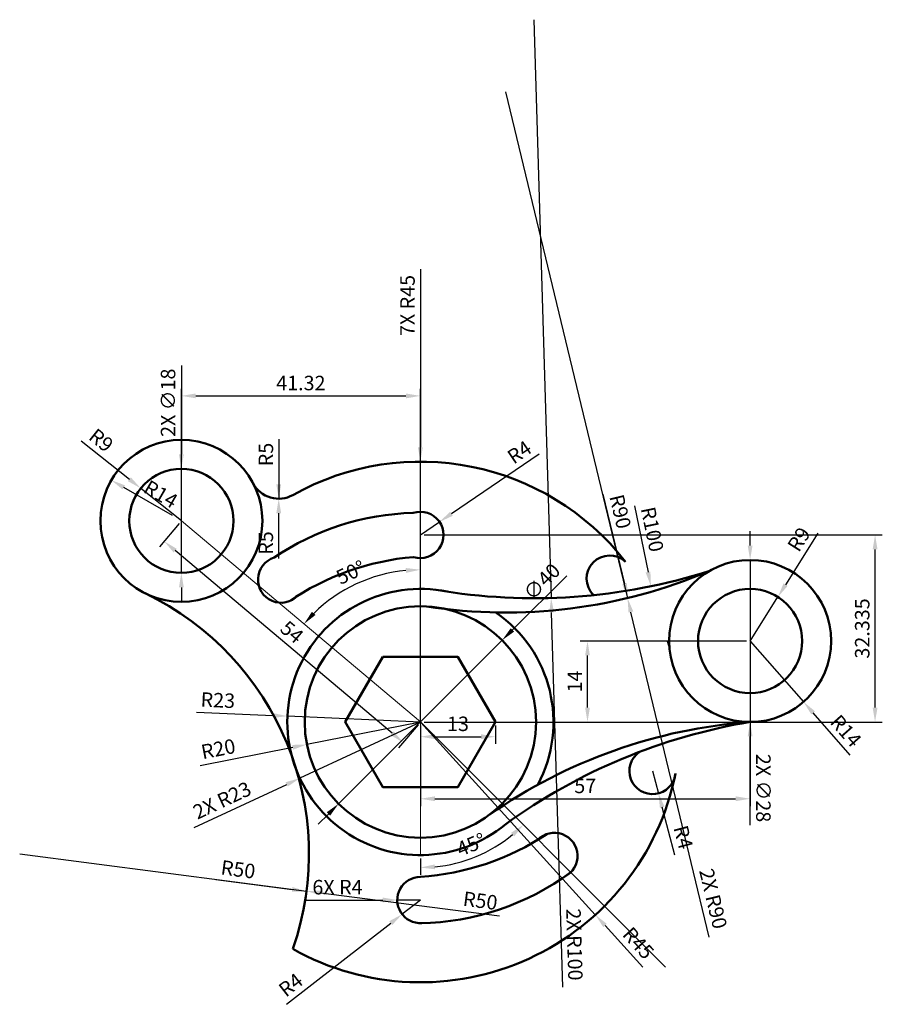
# Model space of a CAD drawing. Units: millimetres. Extents: x 2630 to 2779, y 1501 to 1671.
import ezdxf

# ---------------------------------------------------------------- set-up
doc = ezdxf.new("R2010")
doc.units = ezdxf.units.MM
for name, color, linetype, lineweight in [('M-CONS', 8, 'Continuous', 18), ('M-DIMS', 2, 'Continuous', 25), ('M-OUTL', 7, 'Continuous', 50)]:
    doc.layers.add(name, color=color, linetype=linetype, lineweight=lineweight)
doc.styles.get("Standard").update_dxf_attribs({"font": 'arial.ttf'})
doc.dimstyles.new('ISO-25', dxfattribs={"dimtxt": 2.5, "dimasz": 2.5, "dimexe": 1.25, "dimexo": 0.625, "dimtad": 1, "dimtxsty": 'Standard', "dimcen": 2.5, "dimadec": 0, "dimazin": 0, "dimtfac": 1, "dimtmove": 0, "dimatfit": 3, "dimfxl": 1, "dimarcsym": 0})

# ---------------------------------------------------------------- blocks, each defined once
blk = doc.blocks.new('*D1')
at = {"layer": 'Defpoints', "color": 0, "transparency": 16777216}
for p in [(2658.07, 1584.79), (2655.1, 1581.25), (2699.39, 1550.02)]:
    blk.add_point(p, dxfattribs=at)
at = {"layer": 'M-DIMS', "color": 0, "lineweight": -2, "transparency": 16777216}
for p, q in [((2657.67, 1584.31), (2654.29, 1580.3)), ((2694.5, 1548.09), (2657.01, 1579.64)), ((2698.99, 1549.54), (2695.61, 1545.53))]:
    blk.add_line(p, q, dxfattribs=at)
at = {"layer": 'M-DIMS', "color": 0, "transparency": 16777216}
for points in [[(2657.28, 1579.96), (2656.74, 1579.32), (2655.1, 1581.25)], [(2694.77, 1548.41), (2694.23, 1547.77), (2696.41, 1546.48)]]:
    blk.add_solid(points, dxfattribs=at)
at = {"layer": 'M-DIMS', "color": 0, "transparency": 16777216, "insert": (2676.98, 1565.32), "char_height": 2.5, "attachment_point": 5, "rotation": 319.9171}
blk.add_mtext('54', dxfattribs=at)
blk = doc.blocks.new('*D2')
at = {"layer": 'Defpoints', "color": 0, "transparency": 16777216}
for p in [(2699.39, 1550.02), (2712.39, 1550.02), (2712.39, 1547.48)]:
    blk.add_point(p, dxfattribs=at)
at = {"layer": 'M-DIMS', "color": 0, "lineweight": -2, "transparency": 16777216}
for p, q in [((2699.39, 1549.4), (2699.39, 1546.23)), ((2712.39, 1549.4), (2712.39, 1546.23)), ((2701.89, 1547.48), (2709.89, 1547.48))]:
    blk.add_line(p, q, dxfattribs=at)
at = {"layer": 'M-DIMS', "color": 0, "transparency": 16777216}
for points in [[(2701.89, 1547.9), (2701.89, 1547.06), (2699.39, 1547.48)], [(2709.89, 1547.9), (2709.89, 1547.06), (2712.39, 1547.48)]]:
    blk.add_solid(points, dxfattribs=at)
at = {"layer": 'M-DIMS', "color": 0, "transparency": 16777216, "insert": (2705.89, 1549.38), "char_height": 2.5, "attachment_point": 5}
blk.add_mtext('13', dxfattribs=at)
blk = doc.blocks.new('*D3')
at = {"layer": 'Defpoints', "color": 0, "transparency": 16777216}
for p in [(2728.28, 1564.02), (2756.39, 1564.02), (2699.39, 1550.02)]:
    blk.add_point(p, dxfattribs=at)
at = {"layer": 'M-DIMS', "color": 0, "lineweight": -2, "transparency": 16777216}
for p, q in [((2755.77, 1564.02), (2727.03, 1564.02)), ((2728.28, 1552.52), (2728.28, 1561.52)), ((2700.02, 1550.02), (2729.53, 1550.02))]:
    blk.add_line(p, q, dxfattribs=at)
at = {"layer": 'M-DIMS', "color": 0, "transparency": 16777216}
for points in [[(2727.86, 1561.52), (2728.69, 1561.52), (2728.28, 1564.02)], [(2727.86, 1552.52), (2728.69, 1552.52), (2728.28, 1550.02)]]:
    blk.add_solid(points, dxfattribs=at)
at = {"layer": 'M-DIMS', "color": 0, "transparency": 16777216, "insert": (2726.4, 1557.02), "char_height": 2.5, "attachment_point": 5, "rotation": 90}
blk.add_mtext('14', dxfattribs=at)
blk = doc.blocks.new('*D4')
at = {"layer": 'Defpoints', "color": 0, "transparency": 16777216}
for p in [(2756.39, 1564.02), (2699.39, 1550.02), (2756.39, 1536.75)]:
    blk.add_point(p, dxfattribs=at)
at = {"layer": 'M-DIMS', "color": 0, "lineweight": -2, "transparency": 16777216}
for p, q in [((2756.39, 1563.4), (2756.39, 1535.5)), ((2699.39, 1549.4), (2699.39, 1535.5)), ((2701.89, 1536.75), (2753.89, 1536.75))]:
    blk.add_line(p, q, dxfattribs=at)
at = {"layer": 'M-DIMS', "color": 0, "transparency": 16777216}
for points in [[(2701.89, 1537.17), (2701.89, 1536.34), (2699.39, 1536.75)], [(2753.89, 1537.17), (2753.89, 1536.34), (2756.39, 1536.75)]]:
    blk.add_solid(points, dxfattribs=at)
at = {"layer": 'M-DIMS', "color": 0, "transparency": 16777216, "insert": (2727.89, 1538.65), "char_height": 2.5, "attachment_point": 5}
blk.add_mtext('57', dxfattribs=at)
blk = doc.blocks.new('*D5')
at = {"layer": 'Defpoints', "color": 0, "transparency": 16777216}
for p in [(2674.9, 1593.61), (2674.9, 1588.61)]:
    blk.add_point(p, dxfattribs=at)
at = {"layer": 'M-DIMS', "color": 0, "lineweight": -2, "transparency": 16777216}
blk.add_line((2674.9, 1598.91), (2674.9, 1591.11), dxfattribs=at)
at = {"layer": 'M-DIMS', "color": 0, "transparency": 16777216}
blk.add_solid([(2674.49, 1591.11), (2675.32, 1591.11), (2674.9, 1588.61)], dxfattribs=at)
at = {"layer": 'M-DIMS', "color": 0, "transparency": 16777216, "insert": (2673.01, 1596.26), "char_height": 2.5, "attachment_point": 5, "rotation": 90}
blk.add_mtext('R5', dxfattribs=at)
blk = doc.blocks.new('*D6')
at = {"layer": 'Defpoints', "color": 0, "transparency": 16777216}
for p in [(2645.97, 1591.82), (2658.07, 1584.79)]:
    blk.add_point(p, dxfattribs=at)
at = {"layer": 'M-DIMS', "color": 0, "lineweight": -2, "transparency": 16777216}
blk.add_line((2656.53, 1585.69), (2648.13, 1590.57), dxfattribs=at)
at = {"layer": 'M-DIMS', "color": 0, "transparency": 16777216}
blk.add_solid([(2648.34, 1590.93), (2647.92, 1590.21), (2645.97, 1591.82)], dxfattribs=at)
at = {"layer": 'M-DIMS', "color": 0, "transparency": 16777216, "insert": (2654.36, 1589.13), "char_height": 2.5, "attachment_point": 5, "rotation": 329.8415}
blk.add_mtext('R14', dxfattribs=at)
blk = doc.blocks.new('*D7')
at = {"layer": 'Defpoints', "color": 0, "transparency": 16777216}
for p in [(2651.05, 1590.41), (2658.07, 1584.79)]:
    blk.add_point(p, dxfattribs=at)
at = {"layer": 'M-DIMS', "color": 0, "lineweight": -2, "transparency": 16777216}
for p, q in [((2640.77, 1598.63), (2649.09, 1591.97)), ((2658.07, 1584.79), (2651.05, 1590.41))]:
    blk.add_line(p, q, dxfattribs=at)
at = {"layer": 'M-DIMS', "color": 0, "transparency": 16777216}
blk.add_solid([(2649.35, 1592.3), (2648.83, 1591.65), (2651.05, 1590.41)], dxfattribs=at)
at = {"layer": 'M-DIMS', "color": 0, "transparency": 16777216, "insert": (2644.02, 1598.47), "char_height": 2.5, "attachment_point": 5, "rotation": 321.3553}
blk.add_mtext('R9', dxfattribs=at)
blk = doc.blocks.new('*D8')
at = {"layer": 'Defpoints', "color": 0, "transparency": 16777216}
for p in [(2676.41, 1551.03), (2699.39, 1550.02)]:
    blk.add_point(p, dxfattribs=at)
at = {"layer": 'M-DIMS', "color": 0, "lineweight": -2, "transparency": 16777216}
for p, q in [((2660.68, 1551.73), (2673.92, 1551.14)), ((2699.39, 1550.02), (2676.41, 1551.03))]:
    blk.add_line(p, q, dxfattribs=at)
at = {"layer": 'M-DIMS', "color": 0, "transparency": 16777216}
blk.add_solid([(2673.93, 1551.56), (2673.9, 1550.73), (2676.41, 1551.03)], dxfattribs=at)
at = {"layer": 'M-DIMS', "color": 0, "transparency": 16777216, "insert": (2664.37, 1553.47), "char_height": 2.5, "attachment_point": 5, "rotation": 357.4769}
blk.add_mtext('R23', dxfattribs=at)
blk = doc.blocks.new('*D9')
at = {"layer": 'Defpoints', "color": 0, "transparency": 16777216}
for p in [(2699.39, 1550.02), (2679.77, 1546.14)]:
    blk.add_point(p, dxfattribs=at)
at = {"layer": 'M-DIMS', "color": 0, "lineweight": -2, "transparency": 16777216}
for p, q in [((2699.39, 1550.02), (2679.77, 1546.14)), ((2661.34, 1542.49), (2677.32, 1545.65))]:
    blk.add_line(p, q, dxfattribs=at)
at = {"layer": 'M-DIMS', "color": 0, "transparency": 16777216}
blk.add_solid([(2677.24, 1546.06), (2677.4, 1545.24), (2679.77, 1546.14)], dxfattribs=at)
at = {"layer": 'M-DIMS', "color": 0, "transparency": 16777216, "insert": (2664.51, 1545.05), "char_height": 2.5, "attachment_point": 5, "rotation": 11.1996}
blk.add_mtext('R20', dxfattribs=at)
blk = doc.blocks.new('*D10')
at = {"layer": 'Defpoints', "color": 0, "transparency": 16777216}
for p in [(2630.13, 1527.22), (2679.71, 1520.75)]:
    blk.add_point(p, dxfattribs=at)
at = {"layer": 'M-DIMS', "color": 0, "lineweight": -2, "transparency": 16777216}
blk.add_line((2664.03, 1522.8), (2677.23, 1521.08), dxfattribs=at)
at = {"layer": 'M-DIMS', "color": 0, "transparency": 16777216}
blk.add_solid([(2677.28, 1521.49), (2677.17, 1520.66), (2679.71, 1520.75)], dxfattribs=at)
at = {"layer": 'M-DIMS', "color": 0, "transparency": 16777216, "insert": (2667.85, 1524.22), "char_height": 2.5, "attachment_point": 5, "rotation": 352.5725}
blk.add_mtext('R50', dxfattribs=at)
blk = doc.blocks.new('*D11')
at = {"layer": 'Defpoints', "color": 0, "transparency": 16777216}
for p in [(2699.39, 1519.25), (2696.24, 1516.79)]:
    blk.add_point(p, dxfattribs=at)
at = {"layer": 'M-DIMS', "color": 0, "lineweight": -2, "transparency": 16777216}
for p, q in [((2699.39, 1519.25), (2696.24, 1516.79)), ((2676.26, 1501.22), (2694.26, 1515.26))]:
    blk.add_line(p, q, dxfattribs=at)
at = {"layer": 'M-DIMS', "color": 0, "transparency": 16777216}
blk.add_solid([(2694.01, 1515.59), (2694.52, 1514.93), (2696.24, 1516.79)], dxfattribs=at)
at = {"layer": 'M-DIMS', "color": 0, "transparency": 16777216, "insert": (2677.18, 1504.32), "char_height": 2.5, "attachment_point": 5, "rotation": 37.934}
blk.add_mtext('R4', dxfattribs=at)
blk = doc.blocks.new('*D12')
at = {"layer": 'Defpoints', "color": 0, "transparency": 16777216}
for p in [(2699.39, 1550.02), (2729.63, 1516.7)]:
    blk.add_point(p, dxfattribs=at)
at = {"layer": 'M-DIMS', "color": 0, "lineweight": -2, "transparency": 16777216}
for p, q in [((2699.39, 1550.02), (2729.63, 1516.7)), ((2737.86, 1507.63), (2731.31, 1514.85))]:
    blk.add_line(p, q, dxfattribs=at)
at = {"layer": 'M-DIMS', "color": 0, "transparency": 16777216}
blk.add_solid([(2731.62, 1515.13), (2731, 1514.57), (2729.63, 1516.7)], dxfattribs=at)
at = {"layer": 'M-DIMS', "color": 0, "transparency": 16777216, "insert": (2736.83, 1511.59), "char_height": 2.5, "attachment_point": 5, "rotation": 312.2246}
blk.add_mtext('R45', dxfattribs=at)
blk = doc.blocks.new('*D13')
at = {"layer": 'Defpoints', "color": 0, "transparency": 16777216}
for p in [(2739.52, 1541.56), (2740.55, 1537.69)]:
    blk.add_point(p, dxfattribs=at)
at = {"layer": 'M-DIMS', "color": 0, "lineweight": -2, "transparency": 16777216}
for p, q in [((2739.52, 1541.56), (2740.55, 1537.69)), ((2743.39, 1527), (2741.19, 1535.27))]:
    blk.add_line(p, q, dxfattribs=at)
at = {"layer": 'M-DIMS', "color": 0, "transparency": 16777216}
blk.add_solid([(2741.59, 1535.38), (2740.79, 1535.17), (2740.55, 1537.69)], dxfattribs=at)
at = {"layer": 'M-DIMS', "color": 0, "transparency": 16777216, "insert": (2744.53, 1530.02), "char_height": 2.5, "attachment_point": 5, "rotation": 284.8756}
blk.add_mtext('R4', dxfattribs=at)
blk = doc.blocks.new('*D14')
at = {"layer": 'Defpoints', "color": 0, "transparency": 16777216}
for p in [(2756.39, 1564.02), (2765.62, 1553.5)]:
    blk.add_point(p, dxfattribs=at)
at = {"layer": 'M-DIMS', "color": 0, "lineweight": -2, "transparency": 16777216}
for p, q in [((2756.39, 1564.02), (2765.62, 1553.5)), ((2773.68, 1544.31), (2767.27, 1551.62))]:
    blk.add_line(p, q, dxfattribs=at)
at = {"layer": 'M-DIMS', "color": 0, "transparency": 16777216}
blk.add_solid([(2767.59, 1551.89), (2766.96, 1551.34), (2765.62, 1553.5)], dxfattribs=at)
at = {"layer": 'M-DIMS', "color": 0, "transparency": 16777216, "insert": (2772.71, 1548.27), "char_height": 2.5, "attachment_point": 5, "rotation": 311.2583}
blk.add_mtext('R14', dxfattribs=at)
blk = doc.blocks.new('*D15')
at = {"layer": 'Defpoints', "color": 0, "transparency": 16777216}
for p in [(2761.19, 1571.64), (2756.39, 1564.02)]:
    blk.add_point(p, dxfattribs=at)
at = {"layer": 'M-DIMS', "color": 0, "lineweight": -2, "transparency": 16777216}
for p, q in [((2768.12, 1582.65), (2762.52, 1573.75)), ((2756.39, 1564.02), (2761.19, 1571.64))]:
    blk.add_line(p, q, dxfattribs=at)
at = {"layer": 'M-DIMS', "color": 0, "transparency": 16777216}
blk.add_solid([(2762.16, 1573.97), (2762.87, 1573.53), (2761.19, 1571.64)], dxfattribs=at)
at = {"layer": 'M-DIMS', "color": 0, "transparency": 16777216, "insert": (2765.1, 1581.43), "char_height": 2.5, "attachment_point": 5, "rotation": 57.809}
blk.add_mtext('R9', dxfattribs=at)
blk = doc.blocks.new('*D16')
at = {"layer": 'Defpoints', "color": 0, "transparency": 16777216}
for p in [(2719.01, 1671.42), (2739.25, 1573.49)]:
    blk.add_point(p, dxfattribs=at)
at = {"layer": 'M-DIMS', "color": 0, "lineweight": -2, "transparency": 16777216}
blk.add_line((2736.38, 1587.36), (2738.74, 1575.94), dxfattribs=at)
at = {"layer": 'M-DIMS', "color": 0, "transparency": 16777216}
blk.add_solid([(2739.15, 1576.02), (2738.33, 1575.86), (2739.25, 1573.49)], dxfattribs=at)
at = {"layer": 'M-DIMS', "color": 0, "transparency": 16777216, "insert": (2739.17, 1583.26), "char_height": 2.5, "attachment_point": 5, "rotation": 281.6796}
blk.add_mtext('R100', dxfattribs=at)
blk = doc.blocks.new('*D17')
at = {"layer": 'Defpoints', "color": 0, "transparency": 16777216}
for p in [(2714.12, 1658.95), (2735.27, 1571.47)]:
    blk.add_point(p, dxfattribs=at)
at = {"layer": 'M-DIMS', "color": 0, "lineweight": -2, "transparency": 16777216}
blk.add_line((2730.94, 1589.38), (2734.68, 1573.9), dxfattribs=at)
at = {"layer": 'M-DIMS', "color": 0, "transparency": 16777216}
blk.add_solid([(2735.09, 1574), (2734.28, 1573.8), (2735.27, 1571.47)], dxfattribs=at)
at = {"layer": 'M-DIMS', "color": 0, "transparency": 16777216, "insert": (2733.64, 1586.32), "char_height": 2.5, "attachment_point": 5, "rotation": 283.5898}
blk.add_mtext('R90', dxfattribs=at)
blk = doc.blocks.new('*D18')
at = {"layer": 'Defpoints', "color": 0, "transparency": 16777216}
for p in [(2702.7, 1584.61), (2699.39, 1582.36)]:
    blk.add_point(p, dxfattribs=at)
at = {"layer": 'M-DIMS', "color": 0, "lineweight": -2, "transparency": 16777216}
for p, q in [((2719.92, 1596.32), (2704.77, 1586.01)), ((2699.39, 1582.36), (2702.7, 1584.61))]:
    blk.add_line(p, q, dxfattribs=at)
at = {"layer": 'M-DIMS', "color": 0, "transparency": 16777216}
blk.add_solid([(2704.53, 1586.36), (2705, 1585.67), (2702.7, 1584.61)], dxfattribs=at)
at = {"layer": 'M-DIMS', "color": 0, "transparency": 16777216, "insert": (2716.69, 1596.39), "char_height": 2.5, "attachment_point": 5, "rotation": 34.2167}
blk.add_mtext('R4', dxfattribs=at)
blk = doc.blocks.new('*D19')
at = {"layer": 'Defpoints', "color": 0, "transparency": 16777216}
for p in [(2658.07, 1584.79), (2691.86, 1575.24), (2699.39, 1573.02), (2699.39, 1561.28), (2699.39, 1550.02)]:
    blk.add_point(p, dxfattribs=at)
at = {"layer": 'M-DIMS', "color": 0, "lineweight": -2, "transparency": 16777216}
blk.add_line((2699.39, 1573.65), (2699.39, 1577.59), dxfattribs=at)
blk.add_arc((2699.39, 1550.02), 26.32, 95.4449, 134.4722, dxfattribs=at)
at = {"layer": 'M-DIMS', "color": 0, "transparency": 16777216}
for points in [[(2696.87, 1576.64), (2696.91, 1575.8), (2699.39, 1576.34)], [(2681.26, 1568.52), (2680.65, 1569.08), (2679.26, 1566.97)]]:
    blk.add_solid(points, dxfattribs=at)
at = {"layer": 'M-DIMS', "color": 0, "transparency": 16777216, "insert": (2687.48, 1575.6), "char_height": 2.5, "attachment_point": 5, "rotation": 24.9586}
blk.add_mtext('50°', dxfattribs=at)
blk = doc.blocks.new('*D20')
at = {"layer": 'Defpoints', "color": 0, "transparency": 16777216}
for p in [(2699.39, 1550.02), (2699.39, 1550.02), (2699.39, 1527.02), (2705.9, 1525.72), (2741.76, 1507.65)]:
    blk.add_point(p, dxfattribs=at)
at = {"layer": 'M-DIMS', "color": 0, "lineweight": -2, "transparency": 16777216}
blk.add_line((2699.39, 1526.4), (2699.39, 1523.61), dxfattribs=at)
blk.add_arc((2699.39, 1550.02), 25.16, 275.6954, 309.3046, dxfattribs=at)
at = {"layer": 'M-DIMS', "color": 0, "transparency": 16777216}
for points in [[(2715.05, 1530.86), (2715.61, 1530.24), (2717.18, 1532.23)], [(2701.91, 1524.57), (2701.87, 1525.4), (2699.39, 1524.86)]]:
    blk.add_solid(points, dxfattribs=at)
at = {"layer": 'M-DIMS', "color": 0, "transparency": 16777216, "insert": (2708.29, 1528.53), "char_height": 2.5, "attachment_point": 5, "rotation": 22.5}
blk.add_mtext('45°', dxfattribs=at)
blk = doc.blocks.new('MOUNTING-EYE-OD28-ID18')
for radius in [14, 9]:
    blk.add_circle((14, 14), radius)
blk = doc.blocks.new('*D22')
at = {"layer": 'Defpoints', "color": 0, "transparency": 16777216}
for p in [(2699.39, 1606.39), (2658.07, 1584.79), (2699.39, 1550.02)]:
    blk.add_point(p, dxfattribs=at)
at = {"layer": 'M-DIMS', "color": 0, "lineweight": -2, "transparency": 16777216}
for p, q in [((2658.07, 1585.42), (2658.07, 1607.64)), ((2699.39, 1550.65), (2699.39, 1607.64)), ((2660.57, 1606.39), (2696.89, 1606.39))]:
    blk.add_line(p, q, dxfattribs=at)
at = {"layer": 'M-DIMS', "color": 0, "transparency": 16777216}
for points in [[(2660.57, 1606.81), (2660.57, 1605.97), (2658.07, 1606.39)], [(2696.89, 1606.81), (2696.89, 1605.97), (2699.39, 1606.39)]]:
    blk.add_solid(points, dxfattribs=at)
at = {"layer": 'M-DIMS', "color": 0, "transparency": 16777216, "insert": (2678.73, 1608.29), "char_height": 2.5, "attachment_point": 5}
blk.add_mtext('41.32', dxfattribs=at)
blk = doc.blocks.new('*D23')
at = {"layer": 'Defpoints', "color": 0, "transparency": 16777216}
for p in [(2699.39, 1582.36), (2777.99, 1582.36), (2699.39, 1550.02)]:
    blk.add_point(p, dxfattribs=at)
at = {"layer": 'M-DIMS', "color": 0, "lineweight": -2, "transparency": 16777216}
for p, q in [((2700.02, 1582.36), (2779.24, 1582.36)), ((2777.99, 1552.52), (2777.99, 1579.86)), ((2700.02, 1550.02), (2779.24, 1550.02))]:
    blk.add_line(p, q, dxfattribs=at)
at = {"layer": 'M-DIMS', "color": 0, "transparency": 16777216}
for points in [[(2777.57, 1579.86), (2778.41, 1579.86), (2777.99, 1582.36)], [(2777.57, 1552.52), (2778.41, 1552.52), (2777.99, 1550.02)]]:
    blk.add_solid(points, dxfattribs=at)
at = {"layer": 'M-DIMS', "color": 0, "transparency": 16777216, "insert": (2776.09, 1566.19), "char_height": 2.5, "attachment_point": 5, "rotation": 90}
blk.add_mtext('32.335', dxfattribs=at)
blk = doc.blocks.new('*D24')
at = {"layer": 'Defpoints', "color": 0, "transparency": 16777216}
for p in [(2699.39, 1595.02), (2699.39, 1550.02)]:
    blk.add_point(p, dxfattribs=at)
at = {"layer": 'M-DIMS', "color": 0, "lineweight": -2, "transparency": 16777216}
for p, q in [((2699.39, 1628.32), (2699.39, 1597.52)), ((2699.39, 1550.02), (2699.39, 1595.02))]:
    blk.add_line(p, q, dxfattribs=at)
at = {"layer": 'M-DIMS', "color": 0, "transparency": 16777216}
blk.add_solid([(2698.97, 1597.52), (2699.81, 1597.52), (2699.39, 1595.02)], dxfattribs=at)
at = {"layer": 'M-DIMS', "color": 0, "transparency": 16777216, "insert": (2697.49, 1622.02), "char_height": 2.5, "attachment_point": 5, "rotation": 89.9997}
blk.add_mtext('7X R45', dxfattribs=at)
blk = doc.blocks.new('*D25')
at = {"layer": 'Defpoints', "color": 0, "transparency": 16777216}
for p in [(2699.39, 1550.02), (2678.55, 1540.3)]:
    blk.add_point(p, dxfattribs=at)
at = {"layer": 'M-DIMS', "color": 0, "lineweight": -2, "transparency": 16777216}
for p, q in [((2699.39, 1550.02), (2678.55, 1540.3)), ((2660.31, 1531.79), (2676.28, 1539.24))]:
    blk.add_line(p, q, dxfattribs=at)
at = {"layer": 'M-DIMS', "color": 0, "transparency": 16777216}
blk.add_solid([(2676.1, 1539.62), (2676.46, 1538.86), (2678.55, 1540.3)], dxfattribs=at)
at = {"layer": 'M-DIMS', "color": 0, "transparency": 16777216, "insert": (2665.24, 1536.19), "char_height": 2.5, "attachment_point": 5, "rotation": 25.0057}
blk.add_mtext('2X R23', dxfattribs=at)
blk = doc.blocks.new('*D26')
at = {"layer": 'Defpoints', "color": 0, "transparency": 16777216}
for p in [(2713.53, 1564.16), (2685.25, 1535.88)]:
    blk.add_point(p, dxfattribs=at)
at = {"layer": 'M-DIMS', "color": 0, "lineweight": -2, "transparency": 16777216}
for p, q in [((2724.68, 1575.31), (2715.3, 1565.93)), ((2685.25, 1535.88), (2713.53, 1564.16)), ((2683.48, 1534.11), (2681.71, 1532.34))]:
    blk.add_line(p, q, dxfattribs=at)
at = {"layer": 'M-DIMS', "color": 0, "transparency": 16777216}
for points in [[(2715.01, 1566.23), (2715.6, 1565.64), (2713.53, 1564.16)], [(2683.19, 1534.41), (2683.78, 1533.82), (2685.25, 1535.88)]]:
    blk.add_solid(points, dxfattribs=at)
at = {"layer": 'M-DIMS', "color": 0, "transparency": 16777216, "insert": (2720.62, 1574.04), "char_height": 2.5, "attachment_point": 5, "rotation": 45.0001}
blk.add_mtext('∅40', dxfattribs=at)
blk = doc.blocks.new('*D27')
at = {"layer": 'Defpoints', "color": 0, "transparency": 16777216}
for p in [(2756.39, 1578.02), (2756.39, 1550.02)]:
    blk.add_point(p, dxfattribs=at)
at = {"layer": 'M-DIMS', "color": 0, "lineweight": -2, "transparency": 16777216}
for p, q in [((2756.39, 1580.52), (2756.39, 1583.02)), ((2756.39, 1578.02), (2756.39, 1550.02)), ((2756.39, 1532.18), (2756.39, 1547.52))]:
    blk.add_line(p, q, dxfattribs=at)
at = {"layer": 'M-DIMS', "color": 0, "transparency": 16777216}
for points in [[(2756.81, 1580.52), (2755.97, 1580.52), (2756.39, 1578.02)], [(2756.81, 1547.52), (2755.97, 1547.52), (2756.39, 1550.02)]]:
    blk.add_solid(points, dxfattribs=at)
at = {"layer": 'M-DIMS', "color": 0, "transparency": 16777216, "insert": (2758.36, 1538.6), "char_height": 2.5, "attachment_point": 5, "rotation": 270.0009}
blk.add_mtext('2X ∅28', dxfattribs=at)
blk = doc.blocks.new('*D28')
at = {"layer": 'Defpoints', "color": 0, "transparency": 16777216}
for p in [(2658.07, 1593.79), (2658.07, 1575.79)]:
    blk.add_point(p, dxfattribs=at)
at = {"layer": 'M-DIMS', "color": 0, "lineweight": -2, "transparency": 16777216}
for p, q in [((2658.08, 1611.63), (2658.07, 1596.29)), ((2658.07, 1575.79), (2658.07, 1593.79)), ((2658.07, 1573.29), (2658.07, 1570.79))]:
    blk.add_line(p, q, dxfattribs=at)
at = {"layer": 'M-DIMS', "color": 0, "transparency": 16777216}
for points in [[(2657.66, 1596.29), (2658.49, 1596.29), (2658.07, 1593.79)], [(2657.66, 1573.29), (2658.49, 1573.29), (2658.07, 1575.79)]]:
    blk.add_solid(points, dxfattribs=at)
at = {"layer": 'M-DIMS', "color": 0, "transparency": 16777216, "insert": (2656.1, 1605.21), "char_height": 2.5, "attachment_point": 5, "rotation": 89.9978}
blk.add_mtext('2X ∅18', dxfattribs=at)
blk = doc.blocks.new('*D29')
at = {"layer": 'Defpoints', "color": 0, "transparency": 16777216}
for p in [(2674.9, 1593.61), (2674.9, 1588.61)]:
    blk.add_point(p, dxfattribs=at)
at = {"layer": 'M-DIMS', "color": 0, "lineweight": -2, "transparency": 16777216}
for p, q in [((2674.9, 1593.61), (2674.9, 1588.61)), ((2674.9, 1578.31), (2674.9, 1586.11))]:
    blk.add_line(p, q, dxfattribs=at)
at = {"layer": 'M-DIMS', "color": 0, "transparency": 16777216}
blk.add_solid([(2674.48, 1586.11), (2675.32, 1586.11), (2674.9, 1588.61)], dxfattribs=at)
at = {"layer": 'M-DIMS', "color": 0, "transparency": 16777216, "insert": (2673, 1580.96), "char_height": 2.5, "attachment_point": 5, "rotation": 89.974}
blk.add_mtext('R5', dxfattribs=at)
blk = doc.blocks.new('*D30')
at = {"layer": 'Defpoints', "color": 0, "transparency": 16777216}
for p in [(2695.39, 1519.25), (2699.39, 1519.25)]:
    blk.add_point(p, dxfattribs=at)
at = {"layer": 'M-DIMS', "color": 0, "lineweight": -2, "transparency": 16777216}
for p, q in [((2679.73, 1519.24), (2692.89, 1519.25)), ((2699.39, 1519.25), (2695.39, 1519.25))]:
    blk.add_line(p, q, dxfattribs=at)
at = {"layer": 'M-DIMS', "color": 0, "transparency": 16777216}
blk.add_solid([(2692.89, 1519.67), (2692.89, 1518.83), (2695.39, 1519.25)], dxfattribs=at)
at = {"layer": 'M-DIMS', "color": 0, "transparency": 16777216, "insert": (2685.06, 1521.15), "char_height": 2.5, "attachment_point": 5, "rotation": 0.0337}
blk.add_mtext('6X R4', dxfattribs=at)
blk = doc.blocks.new('*D31')
at = {"layer": 'Defpoints', "color": 0, "transparency": 16777216}
for p in [(2630.13, 1527.22), (2679.71, 1520.79)]:
    blk.add_point(p, dxfattribs=at)
at = {"layer": 'M-DIMS', "color": 0, "lineweight": -2, "transparency": 16777216}
for p, q in [((2630.13, 1527.22), (2679.71, 1520.79)), ((2713.04, 1516.46), (2682.19, 1520.46))]:
    blk.add_line(p, q, dxfattribs=at)
at = {"layer": 'M-DIMS', "color": 0, "transparency": 16777216}
blk.add_solid([(2682.24, 1520.88), (2682.14, 1520.05), (2679.71, 1520.79)], dxfattribs=at)
at = {"layer": 'M-DIMS', "color": 0, "transparency": 16777216, "insert": (2709.71, 1518.81), "char_height": 2.5, "attachment_point": 5, "rotation": 352.6087}
blk.add_mtext('R50', dxfattribs=at)
blk = doc.blocks.new('*D32')
at = {"layer": 'Defpoints', "color": 0, "transparency": 16777216}
for p in [(2714.12, 1658.95), (2735.2, 1571.45)]:
    blk.add_point(p, dxfattribs=at)
at = {"layer": 'M-DIMS', "color": 0, "lineweight": -2, "transparency": 16777216}
for p, q in [((2714.12, 1658.95), (2735.2, 1571.45)), ((2749.33, 1512.82), (2735.79, 1569.02))]:
    blk.add_line(p, q, dxfattribs=at)
at = {"layer": 'M-DIMS', "color": 0, "transparency": 16777216}
blk.add_solid([(2736.19, 1569.12), (2735.38, 1568.93), (2735.2, 1571.45)], dxfattribs=at)
at = {"layer": 'M-DIMS', "color": 0, "transparency": 16777216, "insert": (2749.7, 1519.4), "char_height": 2.5, "attachment_point": 5, "rotation": 283.546}
blk.add_mtext('2X R90', dxfattribs=at)
blk = doc.blocks.new('*D33')
at = {"layer": 'Defpoints', "color": 0, "transparency": 16777216}
for p in [(2719.01, 1671.42), (2722, 1571.47)]:
    blk.add_point(p, dxfattribs=at)
at = {"layer": 'M-DIMS', "color": 0, "lineweight": -2, "transparency": 16777216}
for p, q in [((2719.01, 1671.42), (2722, 1571.47)), ((2724.02, 1504.21), (2722.08, 1568.97))]:
    blk.add_line(p, q, dxfattribs=at)
at = {"layer": 'M-DIMS', "color": 0, "transparency": 16777216}
blk.add_solid([(2722.49, 1568.98), (2721.66, 1568.95), (2722, 1571.47)], dxfattribs=at)
at = {"layer": 'M-DIMS', "color": 0, "transparency": 16777216, "insert": (2725.7, 1511.55), "char_height": 2.5, "attachment_point": 5, "rotation": 271.7166}
blk.add_mtext('2X R100', dxfattribs=at)

msp = doc.modelspace()

# ---------------------------------------------------------------- linework, layer by layer
at = {"layer": 'M-CONS'}
for p, q in [((2699.3908, 1550.0207), (2658.0746, 1584.7911)), ((2699.3908, 1561.2791), (2699.3908, 1573.0207)), ((2699.3908, 1550.0207), (2699.3908, 1564.0207)), ((2699.3908, 1550.0207), (2699.3908, 1527.0207)), ((2699.3908, 1550.0207), (2741.7596, 1507.6519))]:
    msp.add_line(p, q, dxfattribs=at)
at = {"layer": 'M-OUTL'}
msp.add_lwpolyline([(2692.8908, 1561.2791), (2686.3908, 1550.0207), (2692.8908, 1538.7624), (2705.8908, 1538.7624), (2712.3908, 1550.0207), (2705.8908, 1561.2791)], close=True, dxfattribs=at)
msp.add_circle((2699.3908, 1550.0207), 20, dxfattribs=at)
for centre, radius, start, end in [((2699.3908, 1550.0207), 45, 37.976371, 119.325517), ((2674.9023, 1593.6133), 5, 207.666723, 299.325517), ((2699.3908, 1582.3561), 4, 252.540294, 107.910329), ((2699.3276, 1541.1774), 45, 91.485995, 124.100282), ((2675.321, 1574.6313), 4, 107.793138, 316.666592), ((2702.0478, 1533.706), 45, 94.917058, 124.337691), ((2732.1245, 1574.7951), 4, 46.798842, 225.269214), ((2714.1237, 1658.9499), 90, 261.274245, 293.081372), ((2719.0051, 1671.4211), 100, 260.264358, 287.699197), ((2699.3908, 1550.0207), 23, 78.396187, 309.909085), ((2630.1258, 1527.2179), 50, 340.816704, 64.316302), ((2699.3908, 1550.0207), 23, 331.83341, 55.45675), ((2699.3908, 1550.0207), 45, 17.04471, 18.126204), ((2762.9604, 1460.2608), 90, 94.18605, 124.953781), ((2772.7832, 1451.3734), 100, 99.434766, 125.899351), ((2739.5235, 1541.5565), 4, 124.642295, 353.392013), ((2699.3908, 1550.0207), 45, 240.672025, 348.561041), ((2696.3729, 1568.151), 45, 273.845406, 303.57424), ((2722.5418, 1526.8698), 4, 296.202536, 136.032725), ((2698.6455, 1560.2462), 45, 270.949014, 306.432998), ((2699.3908, 1519.2524), 4, 90, 273.529266)]:
    msp.add_arc(centre, radius, start, end, dxfattribs=at)

# ---------------------------------------------------------------- block references
for p in [(2644.0749, 1570.7913), (2742.391, 1550.021)]:
    msp.add_blockref('MOUNTING-EYE-OD28-ID18', p, dxfattribs=at)

# ---------------------------------------------------------------- dimensions: what is measured, and where the dimension line sits
at = {"layer": 'M-DIMS'}
for center, mpoint, override, picture, middle in [((2719.0051, 1671.4211), (2739.2491, 1573.4916), {"dimclrd": 0, "dimclre": 0, "dimclrt": 0}, '*D16', (2737.31, 1582.872)), ((2714.1237, 1658.9499), (2735.2709, 1571.4696), {"dimclrd": 0, "dimclre": 0, "dimclrt": 0}, '*D17', (2731.7896, 1585.8707)), ((2658.0746, 1584.7911), (2651.0453, 1590.4115), {"dimclrd": 0, "dimclre": 0, "dimclrt": 0}, '*D7', (2642.8299, 1596.9802)), ((2674.9023, 1593.6133), (2674.9023, 1588.6133), {"dimclrd": 0, "dimclre": 0, "dimclrt": 0}, '*D5', (2674.9023, 1596.2634)), ((2699.3908, 1582.3561), (2702.6985, 1584.6054), {"dimclrd": 0, "dimclre": 0, "dimclrt": 0}, '*D18', (2717.7434, 1594.8363)), ((2658.0746, 1584.7911), (2645.9697, 1591.8246), {"dimclrd": 0, "dimclre": 0, "dimclrt": 0}, '*D6', (2653.4114, 1587.5006)), ((2756.3908, 1564.0207), (2761.1855, 1571.6372), {"dimclrd": 0, "dimclre": 0, "dimclrt": 0}, '*D15', (2766.7102, 1580.4134)), ((2699.3908, 1550.0207), (2676.4131, 1551.0333), {"dimclrd": 0, "dimclre": 0, "dimclrt": 0}, '*D8', (2664.2895, 1551.5675)), ((2699.3908, 1550.0207), (2679.7717, 1546.1362), {"dimclrd": 0, "dimclre": 0, "dimclrt": 0}, '*D9', (2664.8748, 1543.1866)), ((2739.5235, 1541.5565), (2740.5504, 1537.6905), {"dimclrd": 0, "dimclre": 0, "dimclrt": 0}, '*D13', (2742.7145, 1529.5433)), ((2630.1258, 1527.2179), (2679.7063, 1520.7544), {"dimclrd": 0, "dimclre": 0, "dimclrt": 0}, '*D10', (2667.606, 1522.3318)), ((2630.1258, 1527.2179), (2679.7103, 1520.7857), {"dimdec": 0, "dimlfac": 1, "dimrnd": 0, "dimzin": 0, "dimdsep": 46, "dimlunit": 2}, '*D31', (2709.4611, 1516.9263)), ((2699.3908, 1519.2524), (2696.2359, 1516.7933), {"dimclrd": 0, "dimclre": 0, "dimclrt": 0}, '*D11', (2678.3358, 1502.8414))]:
    dim = msp.add_radius_dim(center=center, mpoint=mpoint, dimstyle='ISO-25', override=override, dxfattribs=at)
    dim.commit()
    dim.dimension.update_dxf_attribs({"geometry": picture, "text_midpoint": middle, "dimtype": 164})
for center, mpoint, text, picture, middle in [((2719.0051, 1671.4211), (2722.0007, 1571.4659), '2X <>', '*D33', (2723.7981, 1511.4929)), ((2714.1237, 1658.9499), (2735.204, 1571.4535), '2X <>', '*D32', (2747.8522, 1518.9556)), ((2699.3908, 1550.0207), (2699.391, 1595.0207), '7X <>', '*D24', (2699.3911, 1622.0207)), ((2699.3908, 1550.0207), (2678.5467, 1540.2984), '2X <>', '*D25', (2666.0402, 1534.4651))]:
    dim = msp.add_radius_dim(center=center, mpoint=mpoint, text=text, dimstyle='ISO-25', override={"dimdec": 0, "dimlfac": 1, "dimrnd": 0, "dimzin": 0, "dimdsep": 46, "dimlunit": 2}, dxfattribs=at)
    dim.commit()
    dim.dimension.update_dxf_attribs({"geometry": picture, "text_midpoint": middle, "dimtype": 164})
dim = msp.add_diameter_dim_2p(p1=(2658.0743, 1575.7911), p2=(2658.075, 1593.7911), text='2X <>', dimstyle='ISO-25', override={"dimdec": 0, "dimlfac": 1, "dimrnd": 0, "dimzin": 0, "dimdsep": 46, "dimlunit": 2}, dxfattribs=at)
dim.commit()
dim.dimension.update_dxf_attribs({"geometry": '*D28', "text_midpoint": (2658.0754, 1605.2099)})
for base, p1, p2, override, picture, middle in [((2699.3908, 1606.3911), (2658.0746, 1584.7911), (2699.3908, 1550.0207), {"dimdec": 2, "dimlfac": 1, "dimrnd": 0, "dimzin": 0, "dimdsep": 46, "dimlunit": 2}, '*D22', (2678.7327, 1608.2934)), ((2756.3908, 1536.7548), (2699.3908, 1550.0207), (2756.3908, 1564.0207), {"dimclrd": 0, "dimclre": 0, "dimclrt": 0}, '*D4', (2727.8908, 1538.6511)), ((2712.3908, 1547.4788), (2699.3908, 1550.0207), (2712.3908, 1550.0207), {"dimclrd": 0, "dimclre": 0, "dimclrt": 0}, '*D2', (2705.8908, 1549.3811))]:
    dim = msp.add_linear_dim(base=base, p1=p1, p2=p2, dimstyle='ISO-25', override=override, dxfattribs=at)
    dim.commit()
    dim.dimension.update_dxf_attribs({"geometry": picture, "text_midpoint": middle})
for center, mpoint, override, picture, middle in [((2674.9023, 1593.6133), (2674.9, 1588.6133), {"dimdec": 0, "dimlfac": 1, "dimrnd": 0, "dimzin": 0, "dimdsep": 46, "dimlunit": 2}, '*D29', (2673.0002, 1580.9641)), ((2756.3908, 1564.0207), (2765.6231, 1553.4963), {"dimclrd": 0, "dimclre": 0, "dimclrt": 0}, '*D14', (2772.7123, 1548.2661)), ((2699.3908, 1550.0207), (2729.6326, 1516.6975), {"dimclrd": 0, "dimclre": 0, "dimclrt": 0}, '*D12', (2736.8306, 1511.5878))]:
    dim = msp.add_radius_dim(center=center, mpoint=mpoint, dimstyle='ISO-25', override=override, dxfattribs=at)
    dim.commit()
    dim.dimension.update_dxf_attribs({"geometry": picture, "text_midpoint": middle})
dim = msp.add_aligned_dim(p1=(2699.3908, 1550.0207), p2=(2658.0746, 1584.7911), distance=4.6236, dimstyle='ISO-25', override={"dimclrd": 0, "dimclre": 0, "dimclrt": 0}, dxfattribs=at)
dim.commit()
dim.dimension.update_dxf_attribs({"geometry": '*D1', "text_midpoint": (2676.9767, 1565.3192)})
for base, line1, line2, picture, middle in [((2691.8552, 1575.2357), ((2699.3908, 1550.0207), (2658.0746, 1584.7911)), ((2699.3908, 1561.2791), (2699.3908, 1573.0207)), '*D19', (2687.4837, 1575.6039)), ((2705.9028, 1525.7177), ((2699.3908, 1550.0207), (2741.7596, 1507.6519)), ((2699.3908, 1550.0207), (2699.3908, 1527.0207)), '*D20', (2708.2936, 1528.5276))]:
    dim = msp.add_angular_dim_2l(base=base, line1=line1, line2=line2, dimstyle='ISO-25', override={"dimclrd": 0, "dimclre": 0, "dimclrt": 0}, dxfattribs=at)
    dim.commit()
    dim.dimension.update_dxf_attribs({"geometry": picture, "text_midpoint": middle})
dim = msp.add_diameter_dim_2p(p1=(2756.3906, 1578.0207), p2=(2756.391, 1550.0207), text='2X <>', dimstyle='ISO-25', override={"dimdec": 0, "dimlfac": 1, "dimrnd": 0, "dimzin": 0, "dimdsep": 46, "dimlunit": 2}, dxfattribs=at)
dim.commit()
dim.dimension.update_dxf_attribs({"geometry": '*D27', "text_midpoint": (2756.3912, 1538.6019), "dimtype": 163})
for base, p2, override, picture, middle in [((2777.9908, 1582.3561), (2699.3908, 1582.3561), {"dimdec": 3, "dimlfac": 1, "dimrnd": 0, "dimzin": 0, "dimdsep": 46, "dimlunit": 2}, '*D23', (2776.0885, 1566.1884)), ((2728.278, 1564.0207), (2756.3908, 1564.0207), {"dimclrd": 0, "dimclre": 0, "dimclrt": 0}, '*D3', (2726.3979, 1557.0207))]:
    dim = msp.add_linear_dim(base=base, p1=(2699.3908, 1550.0207), p2=p2, angle=90, dimstyle='ISO-25', override=override, dxfattribs=at)
    dim.commit()
    dim.dimension.update_dxf_attribs({"geometry": picture, "text_midpoint": middle})
dim = msp.add_diameter_dim_2p(p1=(2685.2487, 1535.8786), p2=(2713.5329, 1564.1629), dimstyle='ISO-25', override={"dimdec": 0, "dimlfac": 1, "dimrnd": 0, "dimzin": 0, "dimdsep": 46, "dimlunit": 2}, dxfattribs=at)
dim.commit()
dim.dimension.update_dxf_attribs({"geometry": '*D26', "text_midpoint": (2722.0182, 1572.6482), "dimtype": 163})
dim = msp.add_radius_dim(center=(2699.3908, 1519.2524), mpoint=(2695.3908, 1519.25), text='6X <>', dimstyle='ISO-25', override={"dimdec": 0, "dimlfac": 1, "dimrnd": 0, "dimzin": 0, "dimdsep": 46, "dimlunit": 2}, dxfattribs=at)
dim.commit()
dim.dimension.update_dxf_attribs({"geometry": '*D30', "text_midpoint": (2685.0614, 1521.1454)})

doc.saveas('drawing.dxf')
